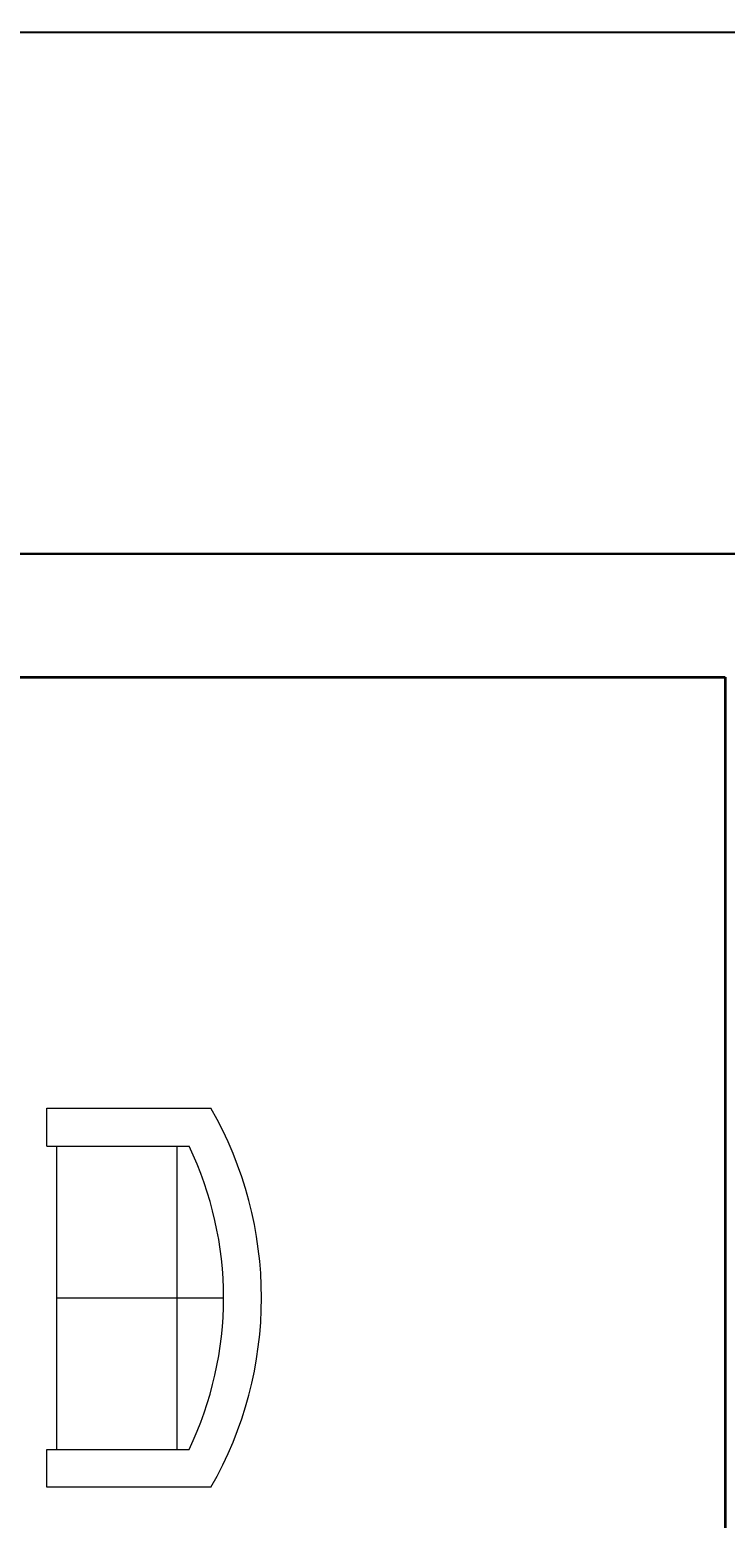
# Model space of a CAD drawing. Units: feet. Extents: x 2219 to 3039, y 1768 to 2369.
# Tile 12 of 16: x 2784 to 2834, y 2261 to 2369. Entities that reach past the tile are written whole.
import ezdxf

# ---------------------------------------------------------------- set-up
doc = ezdxf.new("R2010")
doc.units = ezdxf.units.FT
for name, color, linetype, lineweight in [('A-ANNO-DIMS', 2, 'Continuous', 18), ('A-FURN', 8, 'Continuous', 18), ('A-WALL', 7, 'Continuous', 35), ('C-PROP', 7, 'Continuous', 30)]:
    doc.layers.add(name, color=color, linetype=linetype, lineweight=lineweight)
doc.styles.get("Standard").update_dxf_attribs({"font": 'arial.ttf'})
doc.dimstyles.get("Standard").update_dxf_attribs({"dimtxt": 0.18, "dimasz": 0.18, "dimexe": 0.18, "dimexo": 0.0625, "dimgap": 0.09, "dimtad": 0, "dimtih": 1, "dimtoh": 1, "dimdec": 4, "dimzin": 0, "dimdsep": 46, "dimtxsty": 'Standard', "dimcen": 0.09, "dimadec": 0, "dimazin": 0, "dimtfac": 1, "dimtdec": 4, "dimtofl": 0, "dimtmove": 0, "dimatfit": 3, "dimfxl": 1, "dimtolj": 1, "dimtzin": 0, "dimarcsym": 0})

# ---------------------------------------------------------------- blocks, each defined once
blk = doc.blocks.new('Sofa - Roundback Loveseat 5 ft.')
for p, q in [((0, -32.44198), (0, -5.99998)), ((-24, -33.99998), (-24, -11.46958)), ((24.00004, -33.99998), (24.00004, -11.46958)), ((-23.9998, -13.38178), (23.99986, -13.38178)), ((-24, -32.44198), (24.00004, -32.44198))]:
    blk.add_line(p, q)
for points in [[(-24, -33.99998), (-30, -33.99998), (-30, -7.99998)], [(30.00004, -7.99998), (30.00004, -33.99998), (24.00004, -33.99998)]]:
    blk.add_lwpolyline(points)
for centre, radius, start, end in [((0, -60.24998), 60.24998, 60.13715, 119.8628), ((0, -61.38438), 55.38444, 64.32083, 115.6792)]:
    blk.add_arc(centre, radius, start, end)
blk = doc.blocks.new('*D57')
at = {"layer": 'A-ANNO-DIMS', "color": 0, "lineweight": -2, "transparency": 16777216}
for p, q in [((2782.4, 2330.99), (2782.4, 2369.15)), ((2782.58, 2368.97), (2837.64, 2368.97)), ((2893.22, 2368.97), (2838.16, 2368.97)), ((2893.4, 2330.99), (2893.4, 2369.15))]:
    blk.add_line(p, q, dxfattribs=at)
at = {"layer": 'A-ANNO-DIMS', "color": 0, "transparency": 16777216}
for points in [[(2782.58, 2369), (2782.58, 2368.94), (2782.4, 2368.97)], [(2893.22, 2369), (2893.22, 2368.94), (2893.4, 2368.97)]]:
    blk.add_solid(points, dxfattribs=at)
at = {"layer": 'Defpoints', "color": 0, "transparency": 16777216}
for p in [(2893.4, 2368.97), (2782.4, 2330.92), (2893.4, 2330.92)]:
    blk.add_point(p, dxfattribs=at)
at = {"layer": 'A-ANNO-DIMS', "color": 0, "transparency": 16777216, "insert": (2837.9, 2368.97), "char_height": 0.18, "attachment_point": 5}
blk.add_mtext('\\A1;111', dxfattribs=at)

msp = doc.modelspace()

# ---------------------------------------------------------------- linework, layer by layer
at = {"layer": 'A-WALL'}
for p, q in [((2610.4, 2321.923), (2834.4, 2321.923)), ((2834.4, 2321.923), (2834.4, 2204.687))]:
    msp.add_line(p, q, dxfattribs=at)
at = {"layer": 'C-PROP'}
msp.add_line((2314.4, 2330.923), (3000.4, 2330.923), dxfattribs=at)

# ---------------------------------------------------------------- block references
at = {"layer": 'A-FURN', "xscale": 0.4609193945856732, "yscale": 0.4609193945856732, "zscale": 0.4609193945856732, "rotation": 270}
msp.add_blockref('Sofa - Roundback Loveseat 5 ft.', (2800.552, 2276.63), dxfattribs=at)

# ---------------------------------------------------------------- dimensions: what is measured, and where the dimension line sits
at = {"layer": 'A-ANNO-DIMS'}
dim = msp.add_linear_dim(base=(2893.4, 2368.973), p1=(2782.4, 2330.923), p2=(2893.4, 2330.923), dimstyle='Standard', override={"dimdec": 0, "dimlfac": 1, "dimrnd": 0, "dimzin": 0, "dimdsep": 46, "dimlunit": 2}, dxfattribs=at)
dim.commit()
dim.dimension.update_dxf_attribs({"geometry": '*D57', "text_midpoint": (2837.9, 2368.973)})

doc.saveas('drawing.dxf')
